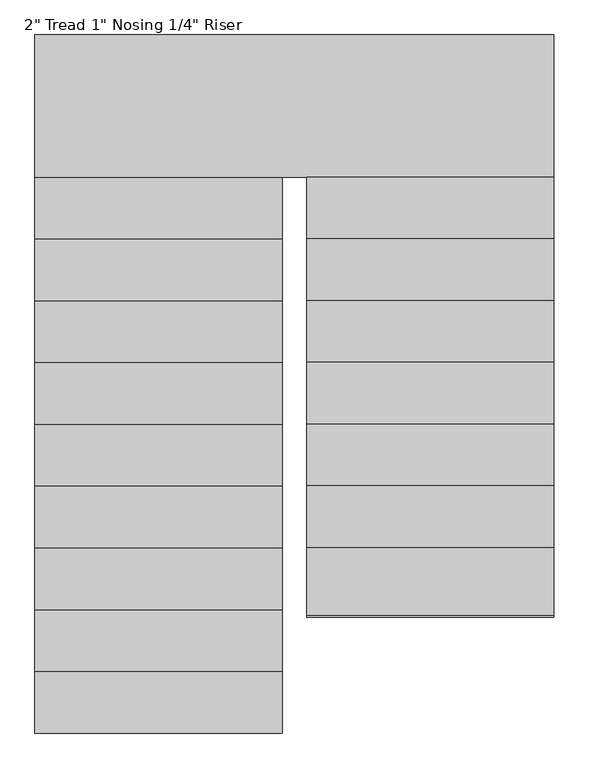
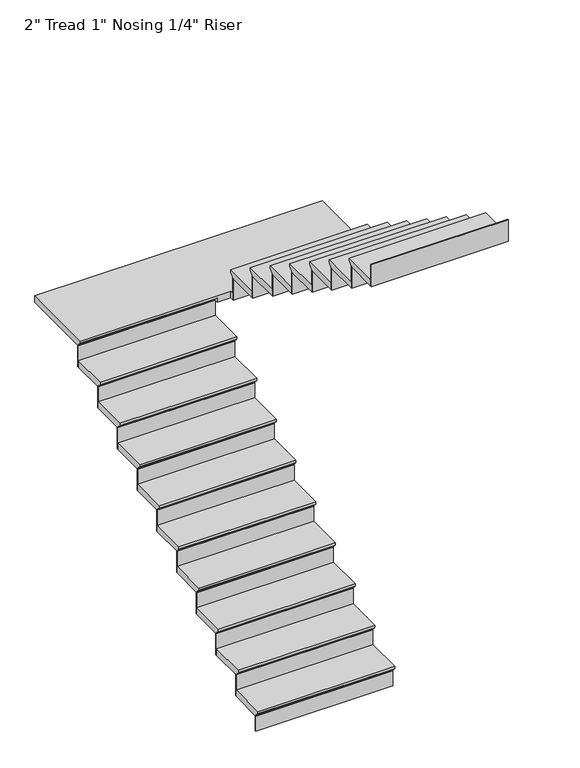
"""IFC4 building model written with IfcOpenShell, lengths in millimetres: stair flight geometry."""

from ifc_helpers import new_model, si_unit, origin, place, context, project, spatial, faceted_brep, source, transform, mapped, element, save


def stair_flight_5c93b7ad(model_context):
    return source(origin(), model_context, "Body", "Brep", [
        faceted_brep([(-8657.8672301, -3404.4302427, 3503.0833333), (-8657.8672301, -3404.4302427, 3522.1333333), (-9673.8672301, -3404.4302427, 3522.1333333), (-9673.8672301, -3404.4302427, 3503.0833333), (-8657.8672301, -3379.0302427, 3477.6833333), (-9673.8672301, -3379.0302427, 3477.6833333), (-8657.8672301, -3125.0302427, 3522.1333333), (-9673.8672301, -3125.0302427, 3522.1333333), (-9673.8672301, -3379.0302427, 3471.3333333), (-9673.8672301, -3125.0302427, 3471.3333333), (-8657.8672301, -3125.0302427, 3471.3333333), (-8657.8672301, -3379.0302427, 3471.3333333)], [[[0, 1, 2, 3]], [[4, 0, 3, 5]], [[2, 1, 6, 7]], [[8, 9, 10, 11]], [[2, 7, 9, 8, 5, 3]], [[8, 11, 4, 5]], [[6, 1, 0, 4, 11, 10]], [[7, 6, 10, 9]]]),
        faceted_brep([(-8657.8672301, -3379.0302427, 3471.3333333), (-8657.8672301, -3379.0302427, 3352.8), (-8657.8672301, -3372.6802427, 3352.8), (-8657.8672301, -3372.6802427, 3471.3333333), (-9673.8672301, -3379.0302427, 3471.3333333), (-9673.8672301, -3372.6802427, 3471.3333333), (-9673.8672301, -3372.6802427, 3352.8), (-9673.8672301, -3379.0302427, 3352.8)], [[[0, 1, 2, 3]], [[4, 5, 6, 7]], [[1, 0, 4, 7]], [[2, 1, 7, 6]], [[3, 2, 6, 5]], [[0, 3, 5, 4]]]),
        faceted_brep([(-8657.8672301, -3125.0302427, 3640.6666667), (-8657.8672301, -3125.0302427, 3471.3333333), (-8657.8672301, -3118.6802427, 3471.3333333), (-8657.8672301, -3118.6802427, 3640.6666667), (-9673.8672301, -3125.0302427, 3640.6666667), (-9673.8672301, -3118.6802427, 3640.6666667), (-9673.8672301, -3118.6802427, 3471.3333333), (-9673.8672301, -3125.0302427, 3471.3333333)], [[[0, 1, 2, 3]], [[4, 5, 6, 7]], [[1, 0, 4, 7]], [[2, 1, 7, 6]], [[3, 2, 6, 5]], [[0, 3, 5, 4]]]),
        faceted_brep([(-9673.8672301, -3150.4302427, 3691.4666667), (-8657.8672301, -3150.4302427, 3691.4666667), (-8657.8672301, -2871.0302427, 3691.4666667), (-9673.8672301, -2871.0302427, 3691.4666667), (-9673.8672301, -3125.0302427, 3640.6666667), (-9673.8672301, -2871.0302427, 3640.6666667), (-8657.8672301, -2871.0302427, 3640.6666667), (-8657.8672301, -3125.0302427, 3640.6666667), (-9673.8672301, -3125.0302427, 3647.0166667), (-9673.8672301, -3150.4302427, 3672.4166667), (-8657.8672301, -3125.0302427, 3647.0166667), (-8657.8672301, -3150.4302427, 3672.4166667)], [[[0, 1, 2, 3]], [[4, 5, 6, 7]], [[0, 3, 5, 4, 8, 9]], [[4, 7, 10, 8]], [[2, 1, 11, 10, 7, 6]], [[3, 2, 6, 5]], [[11, 1, 0, 9]], [[10, 11, 9, 8]]]),
        faceted_brep([(-8657.8672301, -2871.0302427, 3810.0), (-8657.8672301, -2871.0302427, 3640.6666667), (-8657.8672301, -2864.6802427, 3640.6666667), (-8657.8672301, -2864.6802427, 3810.0), (-9673.8672301, -2871.0302427, 3810.0), (-9673.8672301, -2864.6802427, 3810.0), (-9673.8672301, -2864.6802427, 3640.6666667), (-9673.8672301, -2871.0302427, 3640.6666667)], [[[0, 1, 2, 3]], [[4, 5, 6, 7]], [[1, 0, 4, 7]], [[2, 1, 7, 6]], [[3, 2, 6, 5]], [[0, 3, 5, 4]]]),
        faceted_brep([(-9673.8672301, -2896.4302427, 3860.8), (-8657.8672301, -2896.4302427, 3860.8), (-8657.8672301, -2617.0302427, 3860.8), (-9673.8672301, -2617.0302427, 3860.8), (-9673.8672301, -2871.0302427, 3810.0), (-9673.8672301, -2617.0302427, 3810.0), (-8657.8672301, -2617.0302427, 3810.0), (-8657.8672301, -2871.0302427, 3810.0), (-9673.8672301, -2871.0302427, 3816.35), (-9673.8672301, -2896.4302427, 3841.75), (-8657.8672301, -2871.0302427, 3816.35), (-8657.8672301, -2896.4302427, 3841.75)], [[[0, 1, 2, 3]], [[4, 5, 6, 7]], [[0, 3, 5, 4, 8, 9]], [[4, 7, 10, 8]], [[2, 1, 11, 10, 7, 6]], [[3, 2, 6, 5]], [[11, 1, 0, 9]], [[10, 11, 9, 8]]]),
        faceted_brep([(-8657.8672301, -2617.0302427, 3979.3333333), (-8657.8672301, -2617.0302427, 3810.0), (-8657.8672301, -2610.6802427, 3810.0), (-8657.8672301, -2610.6802427, 3979.3333333), (-9673.8672301, -2617.0302427, 3979.3333333), (-9673.8672301, -2610.6802427, 3979.3333333), (-9673.8672301, -2610.6802427, 3810.0), (-9673.8672301, -2617.0302427, 3810.0)], [[[0, 1, 2, 3]], [[4, 5, 6, 7]], [[1, 0, 4, 7]], [[2, 1, 7, 6]], [[3, 2, 6, 5]], [[0, 3, 5, 4]]]),
        faceted_brep([(-9673.8672301, -2642.4302427, 4030.1333333), (-8657.8672301, -2642.4302427, 4030.1333333), (-8657.8672301, -2363.0302427, 4030.1333333), (-9673.8672301, -2363.0302427, 4030.1333333), (-9673.8672301, -2617.0302427, 3979.3333333), (-9673.8672301, -2363.0302427, 3979.3333333), (-8657.8672301, -2363.0302427, 3979.3333333), (-8657.8672301, -2617.0302427, 3979.3333333), (-9673.8672301, -2617.0302427, 3985.6833333), (-9673.8672301, -2642.4302427, 4011.0833333), (-8657.8672301, -2617.0302427, 3985.6833333), (-8657.8672301, -2642.4302427, 4011.0833333)], [[[0, 1, 2, 3]], [[4, 5, 6, 7]], [[0, 3, 5, 4, 8, 9]], [[4, 7, 10, 8]], [[2, 1, 11, 10, 7, 6]], [[3, 2, 6, 5]], [[11, 1, 0, 9]], [[10, 11, 9, 8]]]),
        faceted_brep([(-8657.8672301, -2363.0302427, 4148.6666667), (-8657.8672301, -2363.0302427, 3979.3333333), (-8657.8672301, -2356.6802427, 3979.3333333), (-8657.8672301, -2356.6802427, 4148.6666667), (-9673.8672301, -2363.0302427, 4148.6666667), (-9673.8672301, -2356.6802427, 4148.6666667), (-9673.8672301, -2356.6802427, 3979.3333333), (-9673.8672301, -2363.0302427, 3979.3333333)], [[[0, 1, 2, 3]], [[4, 5, 6, 7]], [[1, 0, 4, 7]], [[2, 1, 7, 6]], [[3, 2, 6, 5]], [[0, 3, 5, 4]]]),
        faceted_brep([(-9673.8672301, -2388.4302427, 4199.4666667), (-8657.8672301, -2388.4302427, 4199.4666667), (-8657.8672301, -2109.0302427, 4199.4666667), (-9673.8672301, -2109.0302427, 4199.4666667), (-9673.8672301, -2363.0302427, 4148.6666667), (-9673.8672301, -2109.0302427, 4148.6666667), (-8657.8672301, -2109.0302427, 4148.6666667), (-8657.8672301, -2363.0302427, 4148.6666667), (-9673.8672301, -2363.0302427, 4155.0166667), (-9673.8672301, -2388.4302427, 4180.4166667), (-8657.8672301, -2363.0302427, 4155.0166667), (-8657.8672301, -2388.4302427, 4180.4166667)], [[[0, 1, 2, 3]], [[4, 5, 6, 7]], [[0, 3, 5, 4, 8, 9]], [[4, 7, 10, 8]], [[2, 1, 11, 10, 7, 6]], [[3, 2, 6, 5]], [[11, 1, 0, 9]], [[10, 11, 9, 8]]]),
        faceted_brep([(-8657.8672301, -2109.0302427, 4318.0), (-8657.8672301, -2109.0302427, 4148.6666667), (-8657.8672301, -2102.6802427, 4148.6666667), (-8657.8672301, -2102.6802427, 4318.0), (-9673.8672301, -2109.0302427, 4318.0), (-9673.8672301, -2102.6802427, 4318.0), (-9673.8672301, -2102.6802427, 4148.6666667), (-9673.8672301, -2109.0302427, 4148.6666667)], [[[0, 1, 2, 3]], [[4, 5, 6, 7]], [[1, 0, 4, 7]], [[2, 1, 7, 6]], [[3, 2, 6, 5]], [[0, 3, 5, 4]]]),
        faceted_brep([(-9673.8672301, -2134.4302427, 4368.8), (-8657.8672301, -2134.4302427, 4368.8), (-8657.8672301, -1855.0302427, 4368.8), (-9673.8672301, -1855.0302427, 4368.8), (-9673.8672301, -2109.0302427, 4318.0), (-9673.8672301, -1855.0302427, 4318.0), (-8657.8672301, -1855.0302427, 4318.0), (-8657.8672301, -2109.0302427, 4318.0), (-9673.8672301, -2109.0302427, 4324.35), (-9673.8672301, -2134.4302427, 4349.75), (-8657.8672301, -2109.0302427, 4324.35), (-8657.8672301, -2134.4302427, 4349.75)], [[[0, 1, 2, 3]], [[4, 5, 6, 7]], [[0, 3, 5, 4, 8, 9]], [[4, 7, 10, 8]], [[2, 1, 11, 10, 7, 6]], [[3, 2, 6, 5]], [[11, 1, 0, 9]], [[10, 11, 9, 8]]]),
        faceted_brep([(-8657.8672301, -1855.0302427, 4487.3333333), (-8657.8672301, -1855.0302427, 4318.0), (-8657.8672301, -1848.6802427, 4318.0), (-8657.8672301, -1848.6802427, 4487.3333333), (-9673.8672301, -1855.0302427, 4487.3333333), (-9673.8672301, -1848.6802427, 4487.3333333), (-9673.8672301, -1848.6802427, 4318.0), (-9673.8672301, -1855.0302427, 4318.0)], [[[0, 1, 2, 3]], [[4, 5, 6, 7]], [[1, 0, 4, 7]], [[2, 1, 7, 6]], [[3, 2, 6, 5]], [[0, 3, 5, 4]]]),
        faceted_brep([(-9673.8672301, -1880.4302427, 4538.1333333), (-8657.8672301, -1880.4302427, 4538.1333333), (-8657.8672301, -1601.0302427, 4538.1333333), (-9673.8672301, -1601.0302427, 4538.1333333), (-9673.8672301, -1855.0302427, 4487.3333333), (-9673.8672301, -1601.0302427, 4487.3333333), (-8657.8672301, -1601.0302427, 4487.3333333), (-8657.8672301, -1855.0302427, 4487.3333333), (-9673.8672301, -1855.0302427, 4493.6833333), (-9673.8672301, -1880.4302427, 4519.0833333), (-8657.8672301, -1855.0302427, 4493.6833333), (-8657.8672301, -1880.4302427, 4519.0833333)], [[[0, 1, 2, 3]], [[4, 5, 6, 7]], [[0, 3, 5, 4, 8, 9]], [[4, 7, 10, 8]], [[2, 1, 11, 10, 7, 6]], [[3, 2, 6, 5]], [[11, 1, 0, 9]], [[10, 11, 9, 8]]]),
        faceted_brep([(-8657.8672301, -1601.0302427, 4656.6666667), (-8657.8672301, -1601.0302427, 4487.3333333), (-8657.8672301, -1594.6802427, 4487.3333333), (-8657.8672301, -1594.6802427, 4656.6666667), (-9673.8672301, -1601.0302427, 4656.6666667), (-9673.8672301, -1594.6802427, 4656.6666667), (-9673.8672301, -1594.6802427, 4487.3333333), (-9673.8672301, -1601.0302427, 4487.3333333)], [[[0, 1, 2, 3]], [[4, 5, 6, 7]], [[1, 0, 4, 7]], [[2, 1, 7, 6]], [[3, 2, 6, 5]], [[0, 3, 5, 4]]]),
        faceted_brep([(-9673.8672301, -1626.4302427, 4707.4666667), (-8657.8672301, -1626.4302427, 4707.4666667), (-8657.8672301, -1347.0302427, 4707.4666667), (-9673.8672301, -1347.0302427, 4707.4666667), (-9673.8672301, -1601.0302427, 4656.6666667), (-9673.8672301, -1347.0302427, 4656.6666667), (-8657.8672301, -1347.0302427, 4656.6666667), (-8657.8672301, -1601.0302427, 4656.6666667), (-9673.8672301, -1601.0302427, 4663.0166667), (-9673.8672301, -1626.4302427, 4688.4166667), (-8657.8672301, -1601.0302427, 4663.0166667), (-8657.8672301, -1626.4302427, 4688.4166667)], [[[0, 1, 2, 3]], [[4, 5, 6, 7]], [[0, 3, 5, 4, 8, 9]], [[4, 7, 10, 8]], [[2, 1, 11, 10, 7, 6]], [[3, 2, 6, 5]], [[11, 1, 0, 9]], [[10, 11, 9, 8]]]),
        faceted_brep([(-8657.8672301, -1347.0302427, 4826.0), (-8657.8672301, -1347.0302427, 4656.6666667), (-8657.8672301, -1340.6802427, 4656.6666667), (-8657.8672301, -1340.6802427, 4826.0), (-9673.8672301, -1347.0302427, 4826.0), (-9673.8672301, -1340.6802427, 4826.0), (-9673.8672301, -1340.6802427, 4656.6666667), (-9673.8672301, -1347.0302427, 4656.6666667)], [[[0, 1, 2, 3]], [[4, 5, 6, 7]], [[1, 0, 4, 7]], [[2, 1, 7, 6]], [[3, 2, 6, 5]], [[0, 3, 5, 4]]]),
        faceted_brep([(-9673.8672301, -1372.4302427, 4876.8), (-8657.8672301, -1372.4302427, 4876.8), (-8657.8672301, -1093.0302427, 4876.8), (-9673.8672301, -1093.0302427, 4876.8), (-9673.8672301, -1347.0302427, 4826.0), (-9673.8672301, -1093.0302427, 4826.0), (-8657.8672301, -1093.0302427, 4826.0), (-8657.8672301, -1347.0302427, 4826.0), (-9673.8672301, -1347.0302427, 4832.35), (-9673.8672301, -1372.4302427, 4857.75), (-8657.8672301, -1347.0302427, 4832.35), (-8657.8672301, -1372.4302427, 4857.75)], [[[0, 1, 2, 3]], [[4, 5, 6, 7]], [[0, 3, 5, 4, 8, 9]], [[4, 7, 10, 8]], [[2, 1, 11, 10, 7, 6]], [[3, 2, 6, 5]], [[11, 1, 0, 9]], [[10, 11, 9, 8]]]),
        faceted_brep([(-8657.8672301, -1093.0302427, 4995.3333333), (-8657.8672301, -1093.0302427, 4826.0), (-8657.8672301, -1086.6802427, 4826.0), (-8657.8672301, -1086.6802427, 4995.3333333), (-9673.8672301, -1093.0302427, 4995.3333333), (-9673.8672301, -1086.6802427, 4995.3333333), (-9673.8672301, -1086.6802427, 4826.0), (-9673.8672301, -1093.0302427, 4826.0)], [[[0, 1, 2, 3]], [[4, 5, 6, 7]], [[1, 0, 4, 7]], [[2, 1, 7, 6]], [[3, 2, 6, 5]], [[0, 3, 5, 4]]]),
        faceted_brep([(-7540.2672301, -1143.8302427, 5046.1333333), (-7540.2672301, -534.2302427, 5046.1333333), (-9673.8672301, -534.2302427, 5046.1333333), (-9673.8672301, -1118.4302427, 5046.1333333), (-8556.2672301, -1118.4302427, 5046.1333333), (-8556.2672301, -1143.8302427, 5046.1333333), (-7540.2672301, -534.2302427, 4995.3333333), (-7540.2672301, -1143.8302427, 4995.3333333), (-8556.2672301, -1143.8302427, 4995.3333333), (-8556.2672301, -1118.4302427, 4995.3333333), (-8657.8672301, -1118.4302427, 4995.3333333), (-8657.8672301, -1093.0302427, 4995.3333333), (-9673.8672301, -1093.0302427, 4995.3333333), (-9673.8672301, -534.2302427, 4995.3333333), (-9673.8672301, -1093.0302427, 5001.6833333), (-9673.8672301, -1118.4302427, 5027.0833333), (-8657.8672301, -1093.0302427, 5001.6833333), (-8657.8672301, -1118.4302427, 5027.0833333)], [[[0, 1, 2, 3, 4, 5]], [[6, 7, 8, 9, 10, 11, 12, 13]], [[1, 0, 7, 6]], [[2, 1, 6, 13]], [[3, 2, 13, 12, 14, 15]], [[12, 11, 16, 14]], [[11, 10, 17, 16]], [[4, 3, 15, 17, 10, 9]], [[5, 4, 9, 8]], [[0, 5, 8, 7]], [[15, 14, 16, 17]]]),
        faceted_brep([(-8556.2672301, -1143.8302427, 5164.6666667), (-8556.2672301, -1143.8302427, 4995.3333333), (-8556.2672301, -1150.1802427, 4995.3333333), (-8556.2672301, -1150.1802427, 5164.6666667), (-7540.2672301, -1143.8302427, 5164.6666667), (-7540.2672301, -1150.1802427, 5164.6666667), (-7540.2672301, -1150.1802427, 4995.3333333), (-7540.2672301, -1143.8302427, 4995.3333333)], [[[0, 1, 2, 3]], [[4, 5, 6, 7]], [[1, 0, 4, 7]], [[2, 1, 7, 6]], [[3, 2, 6, 5]], [[0, 3, 5, 4]]]),
        faceted_brep([(-7540.2672301, -1118.4302427, 5215.4666667), (-8556.2672301, -1118.4302427, 5215.4666667), (-8556.2672301, -1397.8302427, 5215.4666667), (-7540.2672301, -1397.8302427, 5215.4666667), (-7540.2672301, -1143.8302427, 5164.6666667), (-7540.2672301, -1397.8302427, 5164.6666667), (-8556.2672301, -1397.8302427, 5164.6666667), (-8556.2672301, -1143.8302427, 5164.6666667), (-7540.2672301, -1143.8302427, 5171.0166667), (-7540.2672301, -1118.4302427, 5196.4166667), (-8556.2672301, -1143.8302427, 5171.0166667), (-8556.2672301, -1118.4302427, 5196.4166667)], [[[0, 1, 2, 3]], [[4, 5, 6, 7]], [[0, 3, 5, 4, 8, 9]], [[4, 7, 10, 8]], [[2, 1, 11, 10, 7, 6]], [[3, 2, 6, 5]], [[11, 1, 0, 9]], [[10, 11, 9, 8]]]),
        faceted_brep([(-8556.2672301, -1397.8302427, 5334.0), (-8556.2672301, -1397.8302427, 5164.6666667), (-8556.2672301, -1404.1802427, 5164.6666667), (-8556.2672301, -1404.1802427, 5334.0), (-7540.2672301, -1397.8302427, 5334.0), (-7540.2672301, -1404.1802427, 5334.0), (-7540.2672301, -1404.1802427, 5164.6666667), (-7540.2672301, -1397.8302427, 5164.6666667)], [[[0, 1, 2, 3]], [[4, 5, 6, 7]], [[1, 0, 4, 7]], [[2, 1, 7, 6]], [[3, 2, 6, 5]], [[0, 3, 5, 4]]]),
        faceted_brep([(-7540.2672301, -1372.4302427, 5384.8), (-8556.2672301, -1372.4302427, 5384.8), (-8556.2672301, -1651.8302427, 5384.8), (-7540.2672301, -1651.8302427, 5384.8), (-7540.2672301, -1397.8302427, 5334.0), (-7540.2672301, -1651.8302427, 5334.0), (-8556.2672301, -1651.8302427, 5334.0), (-8556.2672301, -1397.8302427, 5334.0), (-7540.2672301, -1397.8302427, 5340.35), (-7540.2672301, -1372.4302427, 5365.75), (-8556.2672301, -1397.8302427, 5340.35), (-8556.2672301, -1372.4302427, 5365.75)], [[[0, 1, 2, 3]], [[4, 5, 6, 7]], [[0, 3, 5, 4, 8, 9]], [[4, 7, 10, 8]], [[2, 1, 11, 10, 7, 6]], [[3, 2, 6, 5]], [[11, 1, 0, 9]], [[10, 11, 9, 8]]]),
        faceted_brep([(-8556.2672301, -1651.8302427, 5503.3333333), (-8556.2672301, -1651.8302427, 5334.0), (-8556.2672301, -1658.1802427, 5334.0), (-8556.2672301, -1658.1802427, 5503.3333333), (-7540.2672301, -1651.8302427, 5503.3333333), (-7540.2672301, -1658.1802427, 5503.3333333), (-7540.2672301, -1658.1802427, 5334.0), (-7540.2672301, -1651.8302427, 5334.0)], [[[0, 1, 2, 3]], [[4, 5, 6, 7]], [[1, 0, 4, 7]], [[2, 1, 7, 6]], [[3, 2, 6, 5]], [[0, 3, 5, 4]]]),
        faceted_brep([(-7540.2672301, -1626.4302427, 5554.1333333), (-8556.2672301, -1626.4302427, 5554.1333333), (-8556.2672301, -1905.8302427, 5554.1333333), (-7540.2672301, -1905.8302427, 5554.1333333), (-7540.2672301, -1651.8302427, 5503.3333333), (-7540.2672301, -1905.8302427, 5503.3333333), (-8556.2672301, -1905.8302427, 5503.3333333), (-8556.2672301, -1651.8302427, 5503.3333333), (-7540.2672301, -1651.8302427, 5509.6833333), (-7540.2672301, -1626.4302427, 5535.0833333), (-8556.2672301, -1651.8302427, 5509.6833333), (-8556.2672301, -1626.4302427, 5535.0833333)], [[[0, 1, 2, 3]], [[4, 5, 6, 7]], [[0, 3, 5, 4, 8, 9]], [[4, 7, 10, 8]], [[2, 1, 11, 10, 7, 6]], [[3, 2, 6, 5]], [[11, 1, 0, 9]], [[10, 11, 9, 8]]]),
        faceted_brep([(-8556.2672301, -1905.8302427, 5672.6666667), (-8556.2672301, -1905.8302427, 5503.3333333), (-8556.2672301, -1912.1802427, 5503.3333333), (-8556.2672301, -1912.1802427, 5672.6666667), (-7540.2672301, -1905.8302427, 5672.6666667), (-7540.2672301, -1912.1802427, 5672.6666667), (-7540.2672301, -1912.1802427, 5503.3333333), (-7540.2672301, -1905.8302427, 5503.3333333)], [[[0, 1, 2, 3]], [[4, 5, 6, 7]], [[1, 0, 4, 7]], [[2, 1, 7, 6]], [[3, 2, 6, 5]], [[0, 3, 5, 4]]]),
        faceted_brep([(-7540.2672301, -1880.4302427, 5723.4666667), (-8556.2672301, -1880.4302427, 5723.4666667), (-8556.2672301, -2159.8302427, 5723.4666667), (-7540.2672301, -2159.8302427, 5723.4666667), (-7540.2672301, -1905.8302427, 5672.6666667), (-7540.2672301, -2159.8302427, 5672.6666667), (-8556.2672301, -2159.8302427, 5672.6666667), (-8556.2672301, -1905.8302427, 5672.6666667), (-7540.2672301, -1905.8302427, 5679.0166667), (-7540.2672301, -1880.4302427, 5704.4166667), (-8556.2672301, -1905.8302427, 5679.0166667), (-8556.2672301, -1880.4302427, 5704.4166667)], [[[0, 1, 2, 3]], [[4, 5, 6, 7]], [[0, 3, 5, 4, 8, 9]], [[4, 7, 10, 8]], [[2, 1, 11, 10, 7, 6]], [[3, 2, 6, 5]], [[11, 1, 0, 9]], [[10, 11, 9, 8]]]),
        faceted_brep([(-8556.2672301, -2159.8302427, 5842.0), (-8556.2672301, -2159.8302427, 5672.6666667), (-8556.2672301, -2166.1802427, 5672.6666667), (-8556.2672301, -2166.1802427, 5842.0), (-7540.2672301, -2159.8302427, 5842.0), (-7540.2672301, -2166.1802427, 5842.0), (-7540.2672301, -2166.1802427, 5672.6666667), (-7540.2672301, -2159.8302427, 5672.6666667)], [[[0, 1, 2, 3]], [[4, 5, 6, 7]], [[1, 0, 4, 7]], [[2, 1, 7, 6]], [[3, 2, 6, 5]], [[0, 3, 5, 4]]]),
        faceted_brep([(-7540.2672301, -2134.4302427, 5892.8), (-8556.2672301, -2134.4302427, 5892.8), (-8556.2672301, -2413.8302427, 5892.8), (-7540.2672301, -2413.8302427, 5892.8), (-7540.2672301, -2159.8302427, 5842.0), (-7540.2672301, -2413.8302427, 5842.0), (-8556.2672301, -2413.8302427, 5842.0), (-8556.2672301, -2159.8302427, 5842.0), (-7540.2672301, -2159.8302427, 5848.35), (-7540.2672301, -2134.4302427, 5873.75), (-8556.2672301, -2159.8302427, 5848.35), (-8556.2672301, -2134.4302427, 5873.75)], [[[0, 1, 2, 3]], [[4, 5, 6, 7]], [[0, 3, 5, 4, 8, 9]], [[4, 7, 10, 8]], [[2, 1, 11, 10, 7, 6]], [[3, 2, 6, 5]], [[11, 1, 0, 9]], [[10, 11, 9, 8]]]),
        faceted_brep([(-8556.2672301, -2413.8302427, 6011.3333333), (-8556.2672301, -2413.8302427, 5842.0), (-8556.2672301, -2420.1802427, 5842.0), (-8556.2672301, -2420.1802427, 6011.3333333), (-7540.2672301, -2413.8302427, 6011.3333333), (-7540.2672301, -2420.1802427, 6011.3333333), (-7540.2672301, -2420.1802427, 5842.0), (-7540.2672301, -2413.8302427, 5842.0)], [[[0, 1, 2, 3]], [[4, 5, 6, 7]], [[1, 0, 4, 7]], [[2, 1, 7, 6]], [[3, 2, 6, 5]], [[0, 3, 5, 4]]]),
        faceted_brep([(-7540.2672301, -2388.4302427, 6062.1333333), (-8556.2672301, -2388.4302427, 6062.1333333), (-8556.2672301, -2667.8302427, 6062.1333333), (-7540.2672301, -2667.8302427, 6062.1333333), (-7540.2672301, -2413.8302427, 6011.3333333), (-7540.2672301, -2667.8302427, 6011.3333333), (-8556.2672301, -2667.8302427, 6011.3333333), (-8556.2672301, -2413.8302427, 6011.3333333), (-7540.2672301, -2413.8302427, 6017.6833333), (-7540.2672301, -2388.4302427, 6043.0833333), (-8556.2672301, -2413.8302427, 6017.6833333), (-8556.2672301, -2388.4302427, 6043.0833333)], [[[0, 1, 2, 3]], [[4, 5, 6, 7]], [[0, 3, 5, 4, 8, 9]], [[4, 7, 10, 8]], [[2, 1, 11, 10, 7, 6]], [[3, 2, 6, 5]], [[11, 1, 0, 9]], [[10, 11, 9, 8]]]),
        faceted_brep([(-8556.2672301, -2667.8302427, 6180.6666667), (-8556.2672301, -2667.8302427, 6011.3333333), (-8556.2672301, -2674.1802427, 6011.3333333), (-8556.2672301, -2674.1802427, 6180.6666667), (-7540.2672301, -2667.8302427, 6180.6666667), (-7540.2672301, -2674.1802427, 6180.6666667), (-7540.2672301, -2674.1802427, 6011.3333333), (-7540.2672301, -2667.8302427, 6011.3333333)], [[[0, 1, 2, 3]], [[4, 5, 6, 7]], [[1, 0, 4, 7]], [[2, 1, 7, 6]], [[3, 2, 6, 5]], [[0, 3, 5, 4]]]),
        faceted_brep([(-8556.2672301, -2921.8302427, 6350.0), (-8556.2672301, -2921.8302427, 6180.6666667), (-8556.2672301, -2928.1802427, 6180.6666667), (-8556.2672301, -2928.1802427, 6350.0), (-7540.2672301, -2921.8302427, 6350.0), (-7540.2672301, -2928.1802427, 6350.0), (-7540.2672301, -2928.1802427, 6180.6666667), (-7540.2672301, -2921.8302427, 6180.6666667)], [[[0, 1, 2, 3]], [[4, 5, 6, 7]], [[1, 0, 4, 7]], [[2, 1, 7, 6]], [[3, 2, 6, 5]], [[0, 3, 5, 4]]]),
        faceted_brep([(-7540.2672301, -2642.4302427, 6231.4666667), (-8556.2672301, -2642.4302427, 6231.4666667), (-8556.2672301, -2921.8302427, 6231.4666667), (-7540.2672301, -2921.8302427, 6231.4666667), (-7540.2672301, -2667.8302427, 6180.6666667), (-7540.2672301, -2921.8302427, 6180.6666667), (-8556.2672301, -2921.8302427, 6180.6666667), (-8556.2672301, -2667.8302427, 6180.6666667), (-7540.2672301, -2667.8302427, 6187.0166667), (-7540.2672301, -2642.4302427, 6212.4166667), (-8556.2672301, -2667.8302427, 6187.0166667), (-8556.2672301, -2642.4302427, 6212.4166667)], [[[0, 1, 2, 3]], [[4, 5, 6, 7]], [[0, 3, 5, 4, 8, 9]], [[4, 7, 10, 8]], [[2, 1, 11, 10, 7, 6]], [[3, 2, 6, 5]], [[11, 1, 0, 9]], [[10, 11, 9, 8]]]),
    ])


if __name__ == "__main__":
    model = new_model("IFC4")
    model_context = context("Model", 3, world=origin())
    ifc_project = project(units=[si_unit("LENGTHUNIT", "METRE", prefix="MILLI")], contexts=[model_context])
    site = spatial("IfcSite", under=ifc_project)
    building = spatial("IfcBuilding", under=site)
    placement = place(None, origin())
    stair_flight_shape = stair_flight_5c93b7ad(model_context)
    element("IfcStairFlight", 1, ObjectType="2\" Tread 1\" Nosing 1/4\" Riser", at=placement, inside=building, context=model_context, shape_type="MappedRepresentation", body=[
        mapped(stair_flight_shape, transform((0.0, 0.0, 0.0), x_axis=(1.0, 0.0, 0.0), y_axis=(0.0, 1.0, 0.0), z_axis=(0.0, 0.0, 1.0))),
    ])
    save(model, "model.ifc")
